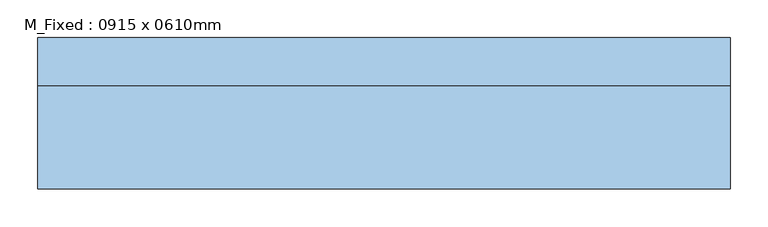
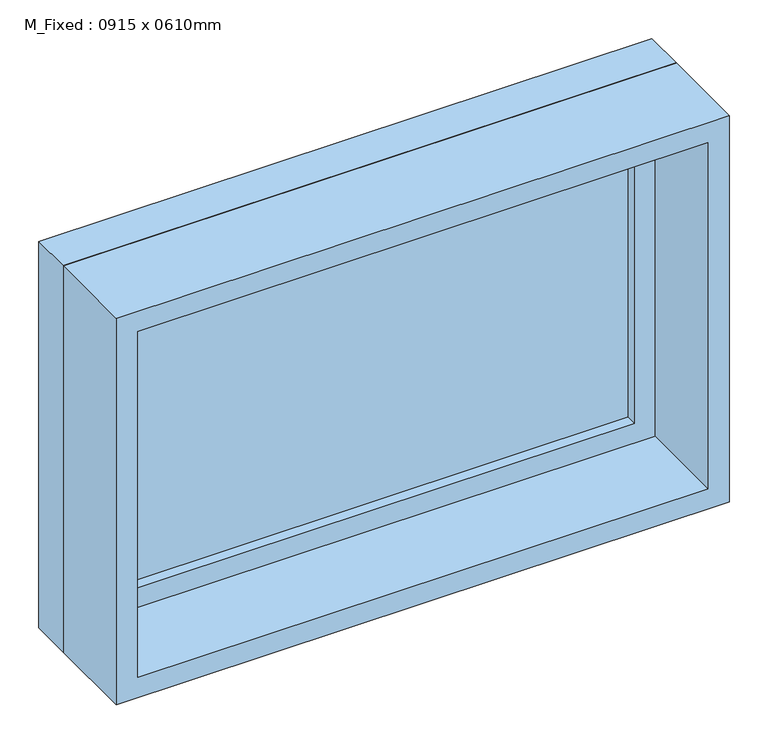
"""IFC4 building model written with IfcOpenShell, lengths in millimetres: window geometry, M_Fixed : 0915 x 0610mm."""

from ifc_helpers import new_model, si_unit, frame, origin, place, context, project, spatial, polyline, outline, extrude, source, transform, mapped, element, save


def m_fixed_0915_x_0610mm_70a843a6(model_context):
    return source(origin(), model_context, "Body", "SweptSolid", [
        extrude(outline(polyline([(-394.5, 78.0), (394.5, 78.0), (394.5, 66.0), (-394.5, 66.0), (-394.5, 78.0)])), frame((0.0, 0.0, 978.0), z_axis=(0.0, 0.0, 1.0), x_axis=(1.0, 0.0, 0.0)), (0.0, 0.0, 1.0), 484.0),
        extrude(outline(polyline([(1506.0, -438.5), (934.0, -438.5), (934.0, 438.5), (1506.0, 438.5), (1506.0, -438.5)]), holes=[polyline([(1462.0, -394.5), (1462.0, 394.5), (978.0, 394.5), (978.0, -394.5), (1462.0, -394.5)])]), frame((0.0, 50.0, 0.0), z_axis=(0.0, 1.0, 0.0), x_axis=(0.0, 0.0, 1.0)), (0.0, 0.0, 1.0), 44.0),
        extrude(outline(polyline([(1525.0, -457.5), (915.0, -457.5), (915.0, 457.5), (1525.0, 457.5), (1525.0, -457.5)]), holes=[polyline([(1506.0, -438.5), (1506.0, 438.5), (934.0, 438.5), (934.0, -438.5), (1506.0, -438.5)])]), frame((0.0, 50.0, 0.0), z_axis=(0.0, 1.0, 0.0), x_axis=(0.0, 0.0, 1.0)), (0.0, 0.0, 1.0), 63.0),
        extrude(outline(polyline([(1525.0, -457.5), (915.0, -457.5), (915.0, 457.5), (1525.0, 457.5), (1525.0, -457.5)]), holes=[polyline([(1493.0, -425.5), (1493.0, 425.5), (947.0, 425.5), (947.0, -425.5), (1493.0, -425.5)])]), frame((0.0, -87.0, 0.0), z_axis=(0.0, 1.0, 0.0), x_axis=(0.0, 0.0, 1.0)), (0.0, 0.0, 1.0), 137.0),
    ])


if __name__ == "__main__":
    model = new_model("IFC4")
    model_context = context("Model", 3, world=origin())
    ifc_project = project(units=[si_unit("LENGTHUNIT", "METRE", prefix="MILLI")], contexts=[model_context])
    site = spatial("IfcSite", under=ifc_project)
    building = spatial("IfcBuilding", under=site)
    placement = place(None, origin())
    m_fixed_0915_x_0610mm_shape = m_fixed_0915_x_0610mm_70a843a6(model_context)
    element("IfcWindow", 1, ObjectType="M_Fixed : 0915 x 0610mm", at=placement, inside=building, context=model_context, shape_type="MappedRepresentation", body=[
        mapped(m_fixed_0915_x_0610mm_shape, transform((0.0, 0.0, 0.0), x_axis=(1.0, 0.0, 0.0), y_axis=(0.0, 1.0, 0.0), z_axis=(0.0, 0.0, 1.0))),
    ])
    save(model, "model.ifc")

# Revit data of these elements
# Type "M_Fixed : 0915 x 0610mm"
#   Type Mark = "14"
#   Height = 2' - 0.01575"
#   Default Sill Height = 3' - 0.02362"
#   Width = 3' - 0.02362"
#   Window Inset = 0' - 0.74803"
#   Frame Exterior Material = Sash
#   Frame Interior Material = Sash
#   Glass Pane Material = Glass
#   Sash = Sash
#   Wall Closure = (empty or 0)
# Element 1 (IfcWindow, "M_Fixed : 0915 x 0610mm")
#   Materials on its faces: "Sash", "Glass"
# Materials
#   "Sash": class "Wood", colour RGB 136 99 55, transparency 0
#   "Glass": class "Glass", colour RGB 218 227 224, transparency 0.85, Description = "Soda Lime Glass", Cost = 0
